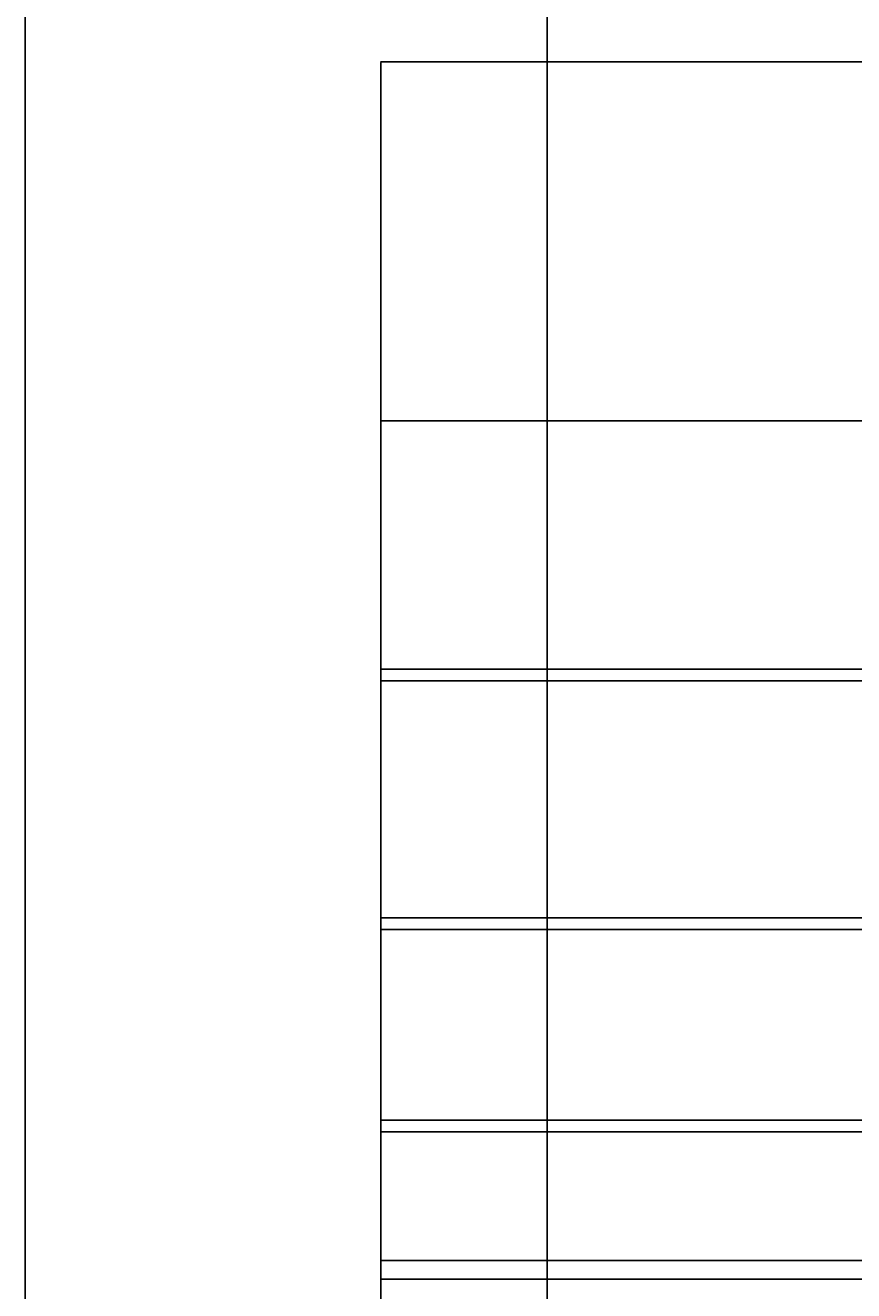
# Model space of a CAD drawing. Units: inches. Extents: x 1770 to 2988, y 1161 to 3221.
# Tile 10 of 44: x 1770 to 2090, y 2032 to 2520. Entities that reach past the tile are written whole.
import ezdxf

# ---------------------------------------------------------------- set-up
doc = ezdxf.new("R2010")
doc.units = ezdxf.units.IN
for name, color, linetype, lineweight in [('A-ANNO-DIMS', 2, 'Continuous', 18), ('A-ANNO-TTLB', 7, 'Continuous', 25), ('C-PROP', 7, 'Continuous', 25)]:
    doc.layers.add(name, color=color, linetype=linetype, lineweight=lineweight)
doc.styles.get("Standard").update_dxf_attribs({"font": 'arial.ttf'})
doc.dimstyles.get("Standard").update_dxf_attribs({"dimtxt": 0.18, "dimasz": 0.18, "dimexe": 0.18, "dimexo": 0.0625, "dimgap": 0.09, "dimtad": 0, "dimtih": 1, "dimtoh": 1, "dimdec": 4, "dimzin": 0, "dimdsep": 46, "dimtxsty": 'Standard', "dimcen": 0.09, "dimadec": 0, "dimazin": 0, "dimtfac": 1, "dimtdec": 4, "dimtofl": 0, "dimtmove": 0, "dimatfit": 3, "dimfxl": 1, "dimtolj": 1, "dimtzin": 0, "dimarcsym": 0})

# ---------------------------------------------------------------- blocks, each defined once
blk = doc.blocks.new('*D56')
at = {"layer": 'A-ANNO-DIMS', "color": 0, "lineweight": -2, "transparency": 16777216}
for p, q in [((1971.53, 2506.34), (1971.53, 2570.7)), ((2802.44, 2506.34), (2802.44, 2570.7)), ((1971.71, 2570.52), (2386.59, 2570.52)), ((2802.26, 2570.52), (2387.38, 2570.52))]:
    blk.add_line(p, q, dxfattribs=at)
at = {"layer": 'A-ANNO-DIMS', "color": 0, "transparency": 16777216}
for points in [[(1971.71, 2570.55), (1971.71, 2570.49), (1971.53, 2570.52)], [(2802.26, 2570.55), (2802.26, 2570.49), (2802.44, 2570.52)]]:
    blk.add_solid(points, dxfattribs=at)
at = {"layer": 'Defpoints', "color": 0, "transparency": 16777216}
for p in [(2802.44, 2570.52), (1971.53, 2506.27), (2802.44, 2506.27)]:
    blk.add_point(p, dxfattribs=at)
at = {"layer": 'A-ANNO-DIMS', "color": 0, "transparency": 16777216, "insert": (2386.99, 2570.52), "char_height": 0.18, "attachment_point": 5}
blk.add_mtext('\\A1;830.9', dxfattribs=at)
blk = doc.blocks.new('*D57')
at = {"layer": 'A-ANNO-DIMS', "color": 0, "lineweight": -2, "transparency": 16777216}
for p, q in [((1971.47, 2506.27), (1907.1, 2506.27)), ((1907.28, 2506.09), (1907.28, 1915.08)), ((1907.28, 1323.71), (1907.28, 1914.72)), ((1971.47, 1323.53), (1907.1, 1323.53))]:
    blk.add_line(p, q, dxfattribs=at)
at = {"layer": 'A-ANNO-DIMS', "color": 0, "transparency": 16777216}
for points in [[(1907.25, 2506.09), (1907.31, 2506.09), (1907.28, 2506.27)], [(1907.25, 1323.71), (1907.31, 1323.71), (1907.28, 1323.53)]]:
    blk.add_solid(points, dxfattribs=at)
at = {"layer": 'Defpoints', "color": 0, "transparency": 16777216}
for p in [(1907.28, 2506.27), (1971.53, 2506.27), (1971.53, 1323.53)]:
    blk.add_point(p, dxfattribs=at)
at = {"layer": 'A-ANNO-DIMS', "color": 0, "transparency": 16777216, "insert": (1907.28, 1914.9), "char_height": 0.18, "attachment_point": 5}
blk.add_mtext('\\A1;1182.7', dxfattribs=at)
blk = doc.blocks.new('*D71')
at = {"layer": 'A-ANNO-DIMS', "color": 0, "lineweight": -2, "transparency": 16777216}
for p, q in [((2160.63, 2171.2), (1907.1, 2171.2)), ((1907.28, 2171.02), (1907.28, 2103.88)), ((1907.28, 2036.38), (1907.28, 2103.52)), ((2160.63, 2036.2), (1907.1, 2036.2))]:
    blk.add_line(p, q, dxfattribs=at)
at = {"layer": 'A-ANNO-DIMS', "color": 0, "transparency": 16777216}
for points in [[(1907.25, 2171.02), (1907.31, 2171.02), (1907.28, 2171.2)], [(1907.25, 2036.38), (1907.31, 2036.38), (1907.28, 2036.2)]]:
    blk.add_solid(points, dxfattribs=at)
at = {"layer": 'Defpoints', "color": 0, "transparency": 16777216}
for p in [(2160.7, 2171.2), (1907.28, 2036.2), (2160.7, 2036.2)]:
    blk.add_point(p, dxfattribs=at)
at = {"layer": 'A-ANNO-DIMS', "color": 0, "transparency": 16777216, "insert": (1907.28, 2103.7), "char_height": 0.18, "attachment_point": 5}
blk.add_mtext('\\A1;135', dxfattribs=at)
blk = doc.blocks.new('*D72')
at = {"layer": 'A-ANNO-DIMS', "color": 0, "lineweight": -2, "transparency": 16777216}
for p, q in [((2456.13, 2267.2), (1907.1, 2267.2)), ((1907.28, 2267.02), (1907.28, 2221.63)), ((1907.28, 2175.88), (1907.28, 2221.27)), ((2456.13, 2175.7), (1907.1, 2175.7))]:
    blk.add_line(p, q, dxfattribs=at)
at = {"layer": 'A-ANNO-DIMS', "color": 0, "transparency": 16777216}
for points in [[(1907.25, 2267.02), (1907.31, 2267.02), (1907.28, 2267.2)], [(1907.25, 2175.88), (1907.31, 2175.88), (1907.28, 2175.7)]]:
    blk.add_solid(points, dxfattribs=at)
at = {"layer": 'Defpoints', "color": 0, "transparency": 16777216}
for p in [(1907.28, 2267.2), (2456.2, 2267.2), (2456.2, 2175.7)]:
    blk.add_point(p, dxfattribs=at)
at = {"layer": 'A-ANNO-DIMS', "color": 0, "transparency": 16777216, "insert": (1907.28, 2221.45), "char_height": 0.18, "attachment_point": 5}
blk.add_mtext('\\A1;91.5', dxfattribs=at)
blk = doc.blocks.new('*D73')
at = {"layer": 'A-ANNO-DIMS', "color": 0, "lineweight": -2, "transparency": 16777216}
for p, q in [((2456.13, 2367.7), (1907.1, 2367.7)), ((1907.28, 2367.52), (1907.28, 2319.88)), ((1907.28, 2271.88), (1907.28, 2319.52)), ((2456.13, 2271.7), (1907.1, 2271.7))]:
    blk.add_line(p, q, dxfattribs=at)
at = {"layer": 'A-ANNO-DIMS', "color": 0, "transparency": 16777216}
for points in [[(1907.25, 2367.52), (1907.31, 2367.52), (1907.28, 2367.7)], [(1907.25, 2271.88), (1907.31, 2271.88), (1907.28, 2271.7)]]:
    blk.add_solid(points, dxfattribs=at)
at = {"layer": 'Defpoints', "color": 0, "transparency": 16777216}
for p in [(1907.28, 2367.7), (2456.2, 2367.7), (2456.2, 2271.7)]:
    blk.add_point(p, dxfattribs=at)
at = {"layer": 'A-ANNO-DIMS', "color": 0, "transparency": 16777216, "insert": (1907.28, 2319.7), "char_height": 0.18, "attachment_point": 5}
blk.add_mtext('\\A1;96', dxfattribs=at)
blk = doc.blocks.new('*D75')
at = {"layer": 'A-ANNO-DIMS', "color": 0, "lineweight": -2, "transparency": 16777216}
for p, q in [((2523.36, 2171.2), (1907.1, 2171.2)), ((1907.28, 2171.02), (1907.28, 2134.56)), ((1907.28, 2097.72), (1907.28, 2134.19)), ((2523.36, 2097.54), (1907.1, 2097.54))]:
    blk.add_line(p, q, dxfattribs=at)
at = {"layer": 'A-ANNO-DIMS', "color": 0, "transparency": 16777216}
for points in [[(1907.25, 2171.02), (1907.31, 2171.02), (1907.28, 2171.2)], [(1907.25, 2097.72), (1907.31, 2097.72), (1907.28, 2097.54)]]:
    blk.add_solid(points, dxfattribs=at)
at = {"layer": 'Defpoints', "color": 0, "transparency": 16777216}
for p in [(2523.42, 2171.2), (1907.28, 2097.54), (2523.42, 2097.54)]:
    blk.add_point(p, dxfattribs=at)
at = {"layer": 'A-ANNO-DIMS', "color": 0, "transparency": 16777216, "insert": (1907.28, 2134.37), "char_height": 0.18, "attachment_point": 5}
blk.add_mtext('\\A1;73.66', dxfattribs=at)
blk = doc.blocks.new('*D88')
at = {"layer": 'A-ANNO-DIMS', "color": 0, "lineweight": -2, "transparency": 16777216}
for p, q in [((2523.36, 2093.04), (1907.1, 2093.04)), ((1907.28, 2092.86), (1907.28, 2068.4)), ((1907.28, 2043.57), (1907.28, 2068.04)), ((2523.36, 2043.39), (1907.1, 2043.39))]:
    blk.add_line(p, q, dxfattribs=at)
at = {"layer": 'A-ANNO-DIMS', "color": 0, "transparency": 16777216}
for points in [[(1907.25, 2092.86), (1907.31, 2092.86), (1907.28, 2093.04)], [(1907.25, 2043.57), (1907.31, 2043.57), (1907.28, 2043.39)]]:
    blk.add_solid(points, dxfattribs=at)
at = {"layer": 'Defpoints', "color": 0, "transparency": 16777216}
for p in [(1907.28, 2093.04), (2523.42, 2093.04), (2523.42, 2043.39)]:
    blk.add_point(p, dxfattribs=at)
at = {"layer": 'A-ANNO-DIMS', "color": 0, "transparency": 16777216, "insert": (1907.28, 2068.22), "char_height": 0.18, "attachment_point": 5}
blk.add_mtext('\\A1;49.65', dxfattribs=at)

msp = doc.modelspace()

# ---------------------------------------------------------------- linework, layer by layer
at = {"layer": 'A-ANNO-TTLB'}
msp.add_lwpolyline([(1769.9155, 3221.2788), (2987.7567, 3221.2788), (2987.7567, 1161.1516), (1769.9155, 1161.1516)], close=True, dxfattribs=at)
at = {"layer": 'C-PROP'}
msp.add_lwpolyline([(1971.5344, 2506.2747), (2802.4374, 2506.2747), (2802.4374, 1323.5288), (1971.5344, 1323.5288)], close=True, dxfattribs=at)

# ---------------------------------------------------------------- dimensions: what is measured, and where the dimension line sits
at = {"layer": 'A-ANNO-DIMS'}
dim = msp.add_linear_dim(base=(2802.4374, 2570.5247), p1=(1971.5344, 2506.2747), p2=(2802.4374, 2506.2747), dimstyle='Standard', override={"dimdec": 1, "dimlfac": 1, "dimrnd": 0, "dimzin": 0, "dimdsep": 46, "dimlunit": 2}, dxfattribs=at)
dim.commit()
dim.dimension.update_dxf_attribs({"geometry": '*D56', "text_midpoint": (2386.9859, 2570.5247)})
for base, p1, p2, override, picture, middle in [((1907.2844, 2506.2747), (1971.5344, 1323.5288), (1971.5344, 2506.2747), {"dimdec": 1, "dimlfac": 1, "dimrnd": 0, "dimzin": 0, "dimdsep": 46, "dimlunit": 2}, '*D57', (1907.2844, 1914.9017)), ((1907.2844, 2367.7021), (2456.196, 2271.7021), (2456.196, 2367.7021), {"dimdec": 0, "dimlfac": 1, "dimrnd": 0, "dimzin": 0, "dimdsep": 46, "dimlunit": 2}, '*D73', (1907.2844, 2319.7021)), ((1907.2844, 2267.2021), (2456.196, 2175.7021), (2456.196, 2267.2021), {"dimdec": 1, "dimlfac": 1, "dimrnd": 0, "dimzin": 0, "dimdsep": 46, "dimlunit": 2}, '*D72', (1907.2844, 2221.4521)), ((1907.2844, 2097.5443), (2523.4179, 2171.2021), (2523.4179, 2097.5443), {"dimdec": 2, "dimlfac": 1, "dimrnd": 0, "dimzin": 0, "dimdsep": 46, "dimlunit": 2}, '*D75', (1907.2844, 2134.3732)), ((1907.2844, 2036.2021), (2160.696, 2171.2021), (2160.696, 2036.2021), {"dimdec": 0, "dimlfac": 1, "dimrnd": 0, "dimzin": 0, "dimdsep": 46, "dimlunit": 2}, '*D71', (1907.2844, 2103.7021)), ((1907.2844, 2093.0443), (2523.4179, 2043.391), (2523.4179, 2093.0443), {"dimdec": 2, "dimlfac": 1, "dimrnd": 0, "dimzin": 0, "dimdsep": 46, "dimlunit": 2}, '*D88', (1907.2844, 2068.2176))]:
    dim = msp.add_linear_dim(base=base, p1=p1, p2=p2, angle=90, dimstyle='Standard', override=override, dxfattribs=at)
    dim.commit()
    dim.dimension.update_dxf_attribs({"geometry": picture, "text_midpoint": middle})

doc.saveas('drawing.dxf')
